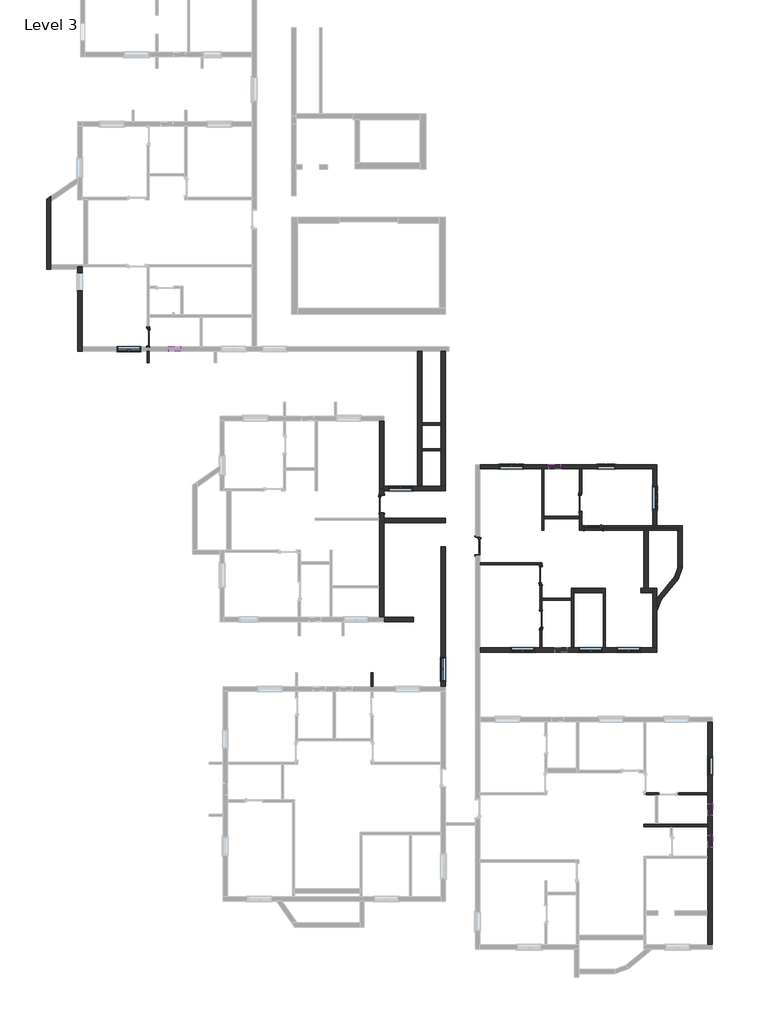
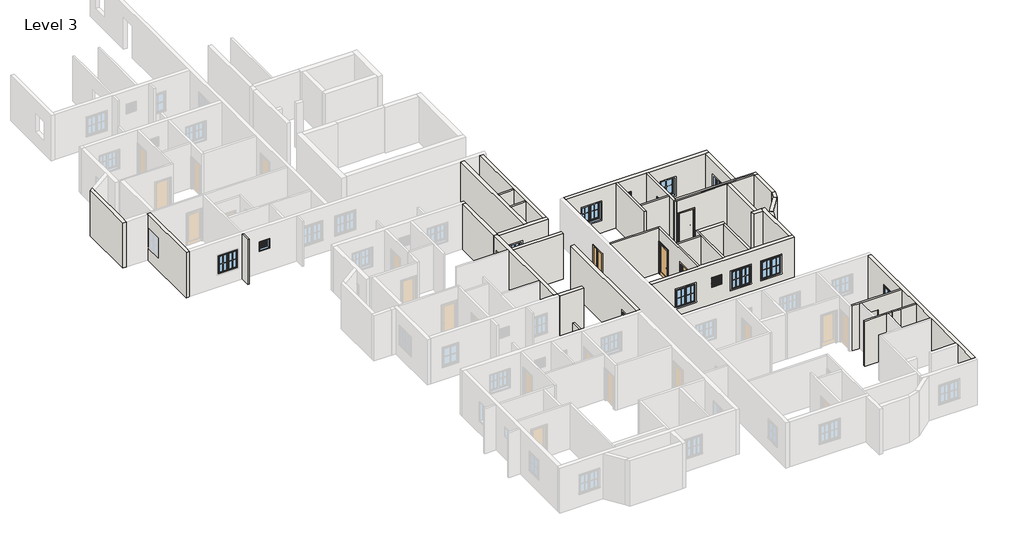
# One storey, part 3 of 7: 39 walls, 15 windows, 7 doors.
# Revit data of these elements (continued)
# Element 52 (IfcWindow, "Window-Casement-Double : 4' x 4'") (continued)
#   Phase Created = New Construction
#   Materials on its faces: "Wood - Stained", "Glass", "Clad - White"
# Element 53 (IfcWindow, "Window-Casement-Double : 4' x 4'")
#   Mark = "44"
#   Window Inset = 0' - 0"
#   Interior Wall Closure = 0' - 2 1/4"
#   Frame Extension = 0' - 0 1/4"
#   Exterior Wall Closure = 0' - 1 1/4"
#   Interior Trim Visibility = yes
#   Exterior Trim Visibility = yes
#   Phase Created = New Construction
#   Materials on its faces: "Wood - Stained", "Glass", "Clad - White"
# Element 54 (IfcWindow, "Window-Casement-Double : 4' x 4'")
#   Mark = "55"
#   Window Inset = 0' - 0"
#   Interior Wall Closure = 0' - 2 1/4"
#   Frame Extension = 0' - 0 1/4"
#   Exterior Wall Closure = 0' - 1 1/4"
#   Interior Trim Visibility = yes
#   Exterior Trim Visibility = yes
#   Phase Created = New Construction
#   Materials on its faces: "Wood - Stained", "Glass", "Clad - White"
# Element 55 (IfcWindow, "Window-Casement-Double : 4' x 4'")
#   Mark = "58"
#   Window Inset = 0' - 0"
#   Interior Wall Closure = 0' - 2 1/4"
#   Frame Extension = 0' - 0 1/4"
#   Exterior Wall Closure = 0' - 1 1/4"
#   Interior Trim Visibility = yes
#   Exterior Trim Visibility = yes
#   Phase Created = New Construction
#   Materials on its faces: "Wood - Stained", "Glass", "Clad - White"
# Element 56 (IfcWindow, "Window-Casement-Double : 4' x 4'")
#   Mark = "63"
#   Window Inset = 0' - 0"
#   Interior Wall Closure = 0' - 2 1/4"
#   Frame Extension = 0' - 0 1/4"
#   Exterior Wall Closure = 0' - 1 1/4"
#   Interior Trim Visibility = yes
#   Exterior Trim Visibility = yes
#   Phase Created = New Construction
#   Materials on its faces: "Wood - Stained", "Glass", "Clad - White"
# Element 57 (IfcWindow, "Window-Louvers : 24\" x 24\"")
#   Mark = "6"
#   Blade Width = 1' - 10 1/2"
#   Phase Created = New Construction
#   Materials on its faces: "Birch"
# Element 58 (IfcWindow, "Window-Louvers : 24\" x 24\"")
#   Mark = "9"
#   Blade Width = 1' - 10 1/2"
#   Phase Created = New Construction
#   Materials on its faces: "Birch"
# Element 59 (IfcWindow, "Window-Louvers : 24\" x 24\"")
#   Mark = "10"
#   Blade Width = 1' - 10 1/2"
#   Phase Created = New Construction
#   Materials on its faces: "Birch"
# Element 60 (IfcWindow, "Window-Louvers : 24\" x 24\"")
#   Mark = "15"
#   Blade Width = 1' - 10 1/2"
#   Phase Created = New Construction
#   Materials on its faces: "Birch"
# Element 61 (IfcWindow, "Window-Louvers : 24\" x 24\"")
#   Mark = "16"
#   Blade Width = 1' - 10 1/2"
#   Phase Created = New Construction
#   Materials on its faces: "Birch"
# Materials
#   "Cherry": class "Wood", colour RGB 226 177 128, transparency 0, Description = "Prunus Serotina", Cost = 0
#   "Aluminum": class "Metal", colour RGB 247 247 247, transparency 0, Description = "Aluminum 6061", Cost = 0
#   "Wood - Stained": class "Wood", colour RGB 224 178 126, transparency 0, Cost = 0
#   "Glass": class "Glass", colour RGB 0 128 192, transparency 0.75, Description = "Soda Lime Glass", Cost = 0
#   "Clad - White": class "Wood", colour RGB 242 242 238, transparency 0, Cost = 0
#   "Birch": class "Wood", colour RGB 224 178 126, transparency 0, Description = "Betula Alleghaniensis", Cost = 0
#   "Default Wall": colour RGB 128 128 128, transparency 0, Cost = 0
